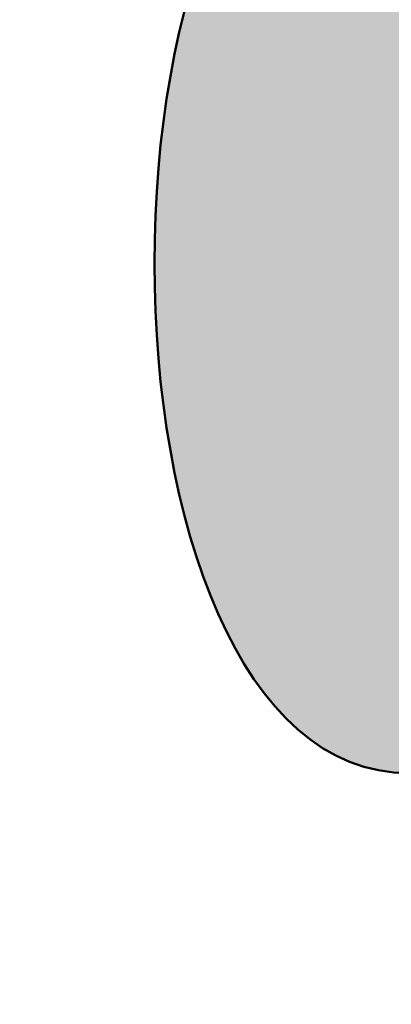
# Model space of a CAD drawing. Units: millimetres. Extents: x 0 to 2267, y 0 to 1823.
# Tile 30 of 256: x 1591.518 to 1593.341, y 1226.115 to 1230.942. Entities that reach past the tile are written whole.
import ezdxf

# ---------------------------------------------------------------- set-up
doc = ezdxf.new("R2010")
doc.units = ezdxf.units.MM
doc.header["$MEASUREMENT"] = 0
doc.layers.add('M-HATC', color=252, linetype='Continuous', lineweight=18)
doc.layers.add('M-OUTL', color=7, linetype='Continuous', lineweight=50)

msp = doc.modelspace()

# ---------------------------------------------------------------- hatches: boundary and pattern name
at = {"layer": 'M-HATC'}
h = msp.add_hatch(color=256, dxfattribs=at)
h.dxf.hatch_style = 1
h.paths.add_polyline_path([(2055.771, 1603.062), (1381.0868, 1603.062), (1381.0868, 1598.062), (2055.771, 1598.062)])
h.paths.add_polyline_path([(2055.771, 1598.062), (1381.0868, 1598.062), (1381.0868, 1593.062), (2055.771, 1593.062)])
h.paths.add_polyline_path([(2051.3074, 1536.7609), (1385.5504, 1536.7609), (1385.5504, 1526.7609), (1387.5504, 1526.7609), (1388.5366, 1525.0528), (1385.3319, 1521.2335), (1385.3319, 1521.2226), (2050.2542, 1522.7491), (2048.3212, 1525.0528), (2049.3074, 1526.7609), (2051.3074, 1526.7609)])
edge = h.paths.add_edge_path()
edge.add_arc((1847.5345, 1379.1492), 135, 222.603061, 222.890851, ccw=False)
edge.add_line((1748.1663, 1287.7656), (1683.0921, 1287.7656))
edge.add_arc((1583.7239, 1379.1492), 135, 317.109149, 317.396939, ccw=False)
edge.add_arc((1678.9686, 1290.6707), 5, 222.8909, 317.1091, ccw=False)
edge.add_arc((1774.2133, 1379.1492), 135, 222.603061, 222.890851, ccw=False)
edge.add_line((1674.8451, 1287.7656), (1609.7709, 1287.7656))
edge.add_arc((1510.4027, 1379.1492), 135, 317.109149, 317.396939, ccw=False)
edge.add_arc((1605.6474, 1290.6707), 5, 222.8909, 317.1091, ccw=False)
edge.add_arc((1700.8921, 1379.1492), 135, 222.603061, 222.890851, ccw=False)
edge.add_line((1601.5239, 1287.7656), (1536.4497, 1287.7656))
edge.add_arc((1437.0815, 1379.1492), 135, 317.109149, 317.396939, ccw=False)
edge.add_arc((1532.3262, 1290.6707), 5, 222.8909, 317.1091, ccw=False)
edge.add_arc((1627.5709, 1379.1492), 135, 222.603061, 222.890851, ccw=False)
edge.add_line((1528.2027, 1287.7656), (1505.9289, 1287.7656))
edge.add_spline(control_points=[(1505.9289, 1287.7656), (1504.2622, 1287.7656), (1504.2622, 1282.7656), (1505.9289, 1282.7656)], knot_values=[0, 0, 0, 0, 5, 5, 5, 5], degree=3, periodic=0)
edge.add_line((1505.9289, 1282.7656), (1930.9289, 1282.7656))
edge.add_spline(control_points=[(1930.9289, 1282.7656), (1932.5956, 1282.7656), (1932.5956, 1287.7656), (1930.9289, 1287.7656)], knot_values=[0, 0, 0, 0, 5, 5, 5, 5], degree=3, periodic=0)
edge.add_line((1930.9289, 1287.7656), (1903.0557, 1287.7656))
edge.add_arc((1803.6875, 1379.1492), 135, 317.109149, 317.396939, ccw=False)
edge.add_arc((1898.9322, 1290.6707), 5, 222.8909, 317.1091, ccw=False)
edge.add_arc((1994.1769, 1379.1492), 135, 222.603061, 222.890851, ccw=False)
edge.add_line((1894.8087, 1287.7656), (1829.7345, 1287.7656))
edge.add_arc((1730.3663, 1379.1492), 135, 317.109149, 317.396939, ccw=False)
edge.add_arc((1825.611, 1290.6707), 5, 222.8909, 317.1091, ccw=False)
edge.add_arc((1920.8557, 1379.1492), 135, 222.603061, 222.890851, ccw=False)
edge.add_line((1821.4875, 1287.7656), (1756.4133, 1287.7656))
edge.add_arc((1657.0451, 1379.1492), 135, 317.109149, 317.396939, ccw=False)
edge.add_arc((1752.2898, 1290.6707), 5, 222.8909, 317.1091, ccw=False)
edge = h.paths.add_edge_path()
edge.add_spline(control_points=[(1843.4289, 1227.2475), (1845.0956, 1227.2475), (1845.0956, 1232.2475), (1843.4289, 1232.2475)], knot_values=[0, 0, 0, 0, 5, 5, 5, 5], degree=3, periodic=0)
edge.add_line((1843.4289, 1232.2475), (1593.4289, 1232.2475))
edge.add_spline(control_points=[(1593.4289, 1232.2475), (1591.7622, 1232.2475), (1591.7622, 1227.2475), (1593.4289, 1227.2475)], knot_values=[0, 0, 0, 0, 5, 5, 5, 5], degree=3, periodic=0)
edge.add_line((1593.4289, 1227.2475), (1843.4289, 1227.2475))
h.paths.add_polyline_path([(1905.9289, 1127.4171), (1530.9289, 1127.4171, 0.414214), (1520.9289, 1117.4171), (1530.9289, 1117.4171), (1915.9289, 1117.4171, 0.414214)])
edge = h.paths.add_edge_path()
edge.add_arc((1397.0858, 1498.4078), 12.7299, 90.78215, 190.87871, ccw=False)
edge.add_line((1396.912, 1511.1365), (1428.0097, 1511.3488))
edge.add_line((1428.0097, 1511.3488), (1433.0097, 1511.3488))
edge.add_line((1433.0097, 1511.3488), (1434.439, 1511.3488))
edge.add_arc((1419.474, 1498.0804), 20, 41.561, 74.08211)
edge.add_line((1424.9592, 1517.3135), (1399.9351, 1517.2561))
edge.add_spline(control_points=[(1399.9307, 1517.2561), (1399.884, 1517.2131), (1399.8328, 1517.1689), (1399.7774, 1517.1236)], knot_values=[11.567499, 11.567499, 11.567499, 11.567499, 11.814249, 11.814249, 11.814249, 11.814249], degree=3, periodic=0)
edge.add_spline(control_points=[(1399.6328, 1517.0099), (1399.5831, 1516.9721), (1399.5307, 1516.9338), (1399.4759, 1516.8947)], knot_values=[11.167718, 11.167718, 11.167718, 11.167718, 11.365188, 11.365188, 11.365188, 11.365188], degree=3, periodic=0)
edge.add_spline(control_points=[(1399.3398, 1516.8001), (1399.1514, 1516.6719), (1398.9384, 1516.5377), (1398.704, 1516.3994)], knot_values=[10.376405, 10.376405, 10.376405, 10.376405, 11.00994, 11.00994, 11.00994, 11.00994], degree=3, periodic=0)
edge.add_spline(control_points=[(1398.6572, 1516.3719), (1398.5789, 1516.326), (1398.4983, 1516.2797), (1398.4155, 1516.2331)], knot_values=[10.125175, 10.125175, 10.125175, 10.125175, 10.334406, 10.334406, 10.334406, 10.334406], degree=3, periodic=0)
edge.add_spline(control_points=[(1398.2642, 1516.1487), (1398.196, 1516.1111), (1398.1263, 1516.0732), (1398.0555, 1516.0351)], knot_values=[9.832246, 9.832246, 9.832246, 9.832246, 9.999658, 9.999658, 9.999658, 9.999658], degree=3, periodic=0)
edge.add_spline(control_points=[(1397.9987, 1516.0048), (1397.7312, 1515.8621), (1397.446, 1515.7171), (1397.1466, 1515.5714)], knot_values=[9.161808, 9.161808, 9.161808, 9.161808, 9.787769, 9.787769, 9.787769, 9.787769], degree=3, periodic=0)
edge.add_spline(control_points=[(1397.1466, 1515.5714), (1396.8418, 1515.423), (1396.5222, 1515.274), (1396.1914, 1515.1262)], knot_values=[8.524455, 8.524455, 8.524455, 8.524455, 9.161808, 9.161808, 9.161808, 9.161808], degree=3, periodic=0)
edge.add_spline(control_points=[(1396.0777, 1515.0756), (1395.9854, 1515.0348), (1395.8922, 1514.994), (1395.7983, 1514.9534)], knot_values=[8.275193, 8.275193, 8.275193, 8.275193, 8.451726, 8.451726, 8.451726, 8.451726], degree=3, periodic=0)
edge.add_spline(control_points=[(1395.6018, 1514.8691), (1395.4997, 1514.8257), (1395.3968, 1514.7824), (1395.2932, 1514.7394)], knot_values=[7.962917, 7.962917, 7.962917, 7.962917, 8.152764, 8.152764, 8.152764, 8.152764], degree=3, periodic=0)
edge.add_spline(control_points=[(1395.2116, 1514.7057), (1394.8278, 1514.5475), (1394.4345, 1514.3929), (1394.0364, 1514.2442)], knot_values=[7.21254, 7.21254, 7.21254, 7.21254, 7.913148, 7.913148, 7.913148, 7.913148], degree=3, periodic=0)
edge.add_spline(control_points=[(1394.0364, 1514.2442), (1393.7076, 1514.1214), (1393.3754, 1514.0027), (1393.0427, 1513.8895)], knot_values=[6.633733, 6.633733, 6.633733, 6.633733, 7.21254, 7.21254, 7.21254, 7.21254], degree=3, periodic=0)
edge.add_spline(control_points=[(1392.8214, 1513.815), (1392.7198, 1513.7812), (1392.6181, 1513.7479), (1392.5166, 1513.7152)], knot_values=[6.328796, 6.328796, 6.328796, 6.328796, 6.505493, 6.505493, 6.505493, 6.505493], degree=3, periodic=0)
edge.add_spline(control_points=[(1392.5166, 1513.7152), (1392.3187, 1513.6515), (1392.1212, 1513.59), (1391.9244, 1513.531)], knot_values=[5.984605, 5.984605, 5.984605, 5.984605, 6.328796, 6.328796, 6.328796, 6.328796], degree=3, periodic=0)
edge.add_spline(control_points=[(1391.7915, 1513.4915), (1391.3122, 1513.3501), (1390.8384, 1513.2239), (1390.3784, 1513.1171)], knot_values=[5.066697, 5.066697, 5.066697, 5.066697, 5.907055, 5.907055, 5.907055, 5.907055], degree=3, periodic=0)
edge.add_spline(control_points=[(1390.3784, 1513.1171), (1390.1797, 1513.071), (1389.9836, 1513.0284), (1389.7907, 1512.9899)], knot_values=[4.70367, 4.70367, 4.70367, 4.70367, 5.066695, 5.066695, 5.066695, 5.066695], degree=3, periodic=0)
edge.add_spline(control_points=[(1389.422, 1512.9204), (1389.2459, 1512.8892), (1389.0729, 1512.8617), (1388.9036, 1512.8381)], knot_values=[4.130571, 4.130571, 4.130571, 4.130571, 4.469816, 4.469816, 4.469816, 4.469816], degree=3, periodic=0)
edge.add_spline(control_points=[(1388.9036, 1512.8381), (1388.591, 1512.7946), (1388.2911, 1512.7644), (1388.0071, 1512.7494)], knot_values=[3.504031, 3.504031, 3.504031, 3.504031, 4.130571, 4.130571, 4.130571, 4.130571], degree=3, periodic=0)
edge.add_spline(control_points=[(1387.9356, 1512.7459), (1387.8538, 1512.7423), (1387.7733, 1512.74), (1387.6944, 1512.739)], knot_values=[3.268866, 3.268866, 3.268866, 3.268866, 3.451164, 3.451164, 3.451164, 3.451164], degree=3, periodic=0)
edge.add_spline(control_points=[(1387.3351, 1512.7443), (1387.2076, 1512.7499), (1387.0847, 1512.7597), (1386.967, 1512.7739)], knot_values=[2.670686, 2.670686, 2.670686, 2.670686, 2.984, 2.984, 2.984, 2.984], degree=3, periodic=0)
edge.add_spline(control_points=[(1386.8327, 1512.7922), (1386.8209, 1512.7941), (1386.8092, 1512.7959), (1386.7975, 1512.7979)], knot_values=[2.516981, 2.516981, 2.516981, 2.516981, 2.549528, 2.549528, 2.549528, 2.549528], degree=3, periodic=0)
edge.add_spline(control_points=[(1386.4526, 1512.8735), (1386.4257, 1512.881), (1386.3993, 1512.889), (1386.3733, 1512.8972)], knot_values=[2.095869, 2.095869, 2.095869, 2.095869, 2.17941, 2.17941, 2.17941, 2.17941], degree=3, periodic=0)
edge.add_spline(control_points=[(1386.0691, 1513.0189), (1386.0634, 1513.0217), (1386.0577, 1513.0246), (1386.052, 1513.0275)], knot_values=[1.72453, 1.72453, 1.72453, 1.72453, 1.745933, 1.745933, 1.745933, 1.745933], degree=3, periodic=0)
edge.add_arc((1399.474, 1498.0804), 20, 131.82432, 180)
edge.add_arc((1630.3336, 1505.5484), 250.9708, 181.705176, 236.427975)
edge.add_arc((1605.3399, 1483.3044), 218.7822, 238.660829, 243.34961)
edge.add_arc((1647.0911, 1510.3592), 262.8986, 183.129836, 237.853442, ccw=False)
h.paths.add_polyline_path([(1406.5369, 1391.9644, 0.149382), (1491.5506, 1296.4418, -0.129517)], flags=17)
edge = h.paths.add_edge_path()
edge.add_arc((2037.3838, 1498.0804), 20, 0, 48.26587)
edge.add_spline(control_points=[(2050.6973, 1513.0052), (2050.6512, 1512.9847), (2050.6034, 1512.9655), (2050.5539, 1512.9477)], knot_values=[1.835652, 1.835652, 1.835652, 1.835652, 2.000781, 2.000781, 2.000781, 2.000781], degree=3, periodic=0)
edge.add_spline(control_points=[(2050.4616, 1512.9166), (2050.479, 1512.9221), (2050.4963, 1512.9277), (2050.5133, 1512.9335)], knot_values=[2.045477, 2.045477, 2.045477, 2.045477, 2.101389, 2.101389, 2.101389, 2.101389], degree=3, periodic=0)
edge.add_spline(control_points=[(2050.129, 1512.8342), (2050.1984, 1512.8473), (2050.2657, 1512.8623), (2050.3308, 1512.8792)], knot_values=[2.237629, 2.237629, 2.237629, 2.237629, 2.435841, 2.435841, 2.435841, 2.435841], degree=3, periodic=0)
edge.add_spline(control_points=[(2050.0946, 1512.8278), (2050.1061, 1512.8299), (2050.1176, 1512.832), (2050.129, 1512.8342)], knot_values=[2.435841, 2.435841, 2.435841, 2.435841, 2.468321, 2.468321, 2.468321, 2.468321], degree=3, periodic=0)
edge.add_spline(control_points=[(2049.7843, 1512.7851), (2049.8552, 1512.7922), (2049.9243, 1512.8008), (2049.9917, 1512.8109)], knot_values=[2.563852, 2.563852, 2.563852, 2.563852, 2.748541, 2.748541, 2.748541, 2.748541], degree=3, periodic=0)
edge.add_spline(control_points=[(2049.4052, 1512.7617), (2049.5364, 1512.7653), (2049.6629, 1512.773), (2049.7843, 1512.7851)], knot_values=[2.748541, 2.748541, 2.748541, 2.748541, 3.064882, 3.064882, 3.064882, 3.064882], degree=3, periodic=0)
edge.add_spline(control_points=[(2049.1698, 1512.7597), (2049.2336, 1512.7591), (2049.2965, 1512.7594), (2049.3584, 1512.7606)], knot_values=[3.102309, 3.102309, 3.102309, 3.102309, 3.2503, 3.2503, 3.2503, 3.2503], degree=3, periodic=0)
edge.add_spline(control_points=[(2048.8573, 1512.7691), (2048.9638, 1512.7638), (2049.068, 1512.7606), (2049.1698, 1512.7597)], knot_values=[3.2503, 3.2503, 3.2503, 3.2503, 3.486069, 3.486069, 3.486069, 3.486069], degree=3, periodic=0)
edge.add_spline(control_points=[(2048.6924, 1512.7789), (2048.3729, 1512.8009), (2048.0345, 1512.8411), (2047.6817, 1512.897)], knot_values=[3.606429, 3.606429, 3.606429, 3.606429, 4.2989, 4.2989, 4.2989, 4.2989], degree=3, periodic=0)
edge.add_spline(control_points=[(2047.6817, 1512.897), (2047.5458, 1512.9185), (2047.4077, 1512.9424), (2047.2678, 1512.9685)], knot_values=[4.2989, 4.2989, 4.2989, 4.2989, 4.565769, 4.565769, 4.565769, 4.565769], degree=3, periodic=0)
edge.add_spline(control_points=[(2047.2678, 1512.9685), (2047.1449, 1512.9914), (2047.0207, 1513.016), (2046.8951, 1513.0422)], knot_values=[4.565769, 4.565769, 4.565769, 4.565769, 4.799971, 4.799971, 4.799971, 4.799971], degree=3, periodic=0)
edge.add_spline(control_points=[(2046.8951, 1513.0422), (2046.5286, 1513.1188), (2046.1513, 1513.209), (2045.7676, 1513.3107)], knot_values=[4.799971, 4.799971, 4.799971, 4.799971, 5.483718, 5.483718, 5.483718, 5.483718], degree=3, periodic=0)
edge.add_spline(control_points=[(2045.7676, 1513.3107), (2045.3724, 1513.4154), (2044.9704, 1513.5322), (2044.5662, 1513.6588)], knot_values=[5.483718, 5.483718, 5.483718, 5.483718, 6.187866, 6.187866, 6.187866, 6.187866], degree=3, periodic=0)
edge.add_spline(control_points=[(2044.5662, 1513.6588), (2044.4149, 1513.7061), (2044.2633, 1513.7549), (2044.1116, 1513.8048)], knot_values=[6.187866, 6.187866, 6.187866, 6.187866, 6.451551, 6.451551, 6.451551, 6.451551], degree=3, periodic=0)
edge.add_spline(control_points=[(2044.1116, 1513.8048), (2043.9967, 1513.8427), (2043.8817, 1513.8813), (2043.7668, 1513.9205)], knot_values=[6.451551, 6.451551, 6.451551, 6.451551, 6.651434, 6.651434, 6.651434, 6.651434], degree=3, periodic=0)
edge.add_spline(control_points=[(2043.7668, 1513.9205), (2043.3716, 1514.0554), (2042.9774, 1514.1979), (2042.5886, 1514.3458)], knot_values=[6.651434, 6.651434, 6.651434, 6.651434, 7.338879, 7.338879, 7.338879, 7.338879], degree=3, periodic=0)
edge.add_spline(control_points=[(2042.5886, 1514.3458), (2042.1643, 1514.5071), (2041.7465, 1514.6749), (2041.3409, 1514.846)], knot_values=[7.338879, 7.338879, 7.338879, 7.338879, 8.089209, 8.089209, 8.089209, 8.089209], degree=3, periodic=0)
edge.add_spline(control_points=[(2041.3409, 1514.846), (2041.1028, 1514.9465), (2040.869, 1515.0481), (2040.6405, 1515.1502)], knot_values=[8.089209, 8.089209, 8.089209, 8.089209, 8.529587, 8.529587, 8.529587, 8.529587], degree=3, periodic=0)
edge.add_spline(control_points=[(2040.51, 1515.2089), (2040.0824, 1515.4022), (2039.6747, 1515.5971), (2039.295, 1515.7894)], knot_values=[8.613818, 8.613818, 8.613818, 8.613818, 9.44571, 9.44571, 9.44571, 9.44571], degree=3, periodic=0)
edge.add_spline(control_points=[(2039.295, 1515.7894), (2039.0618, 1515.9075), (2038.8391, 1516.0246), (2038.6288, 1516.1398)], knot_values=[9.44571, 9.44571, 9.44571, 9.44571, 9.956404, 9.956404, 9.956404, 9.956404], degree=3, periodic=0)
edge.add_spline(control_points=[(2038.6288, 1516.1398), (2038.5187, 1516.2001), (2038.4121, 1516.2598), (2038.309, 1516.3189)], knot_values=[9.956404, 9.956404, 9.956404, 9.956404, 10.223542, 10.223542, 10.223542, 10.223542], degree=3, periodic=0)
edge.add_spline(control_points=[(2038.309, 1516.3189), (2038.2138, 1516.3735), (2038.1216, 1516.4276), (2038.0328, 1516.481)], knot_values=[10.223542, 10.223542, 10.223542, 10.223542, 10.47051, 10.47051, 10.47051, 10.47051], degree=3, periodic=0)
edge.add_spline(control_points=[(2038.0328, 1516.481), (2037.7855, 1516.6296), (2037.5639, 1516.773), (2037.3722, 1516.909)], knot_values=[10.47051, 10.47051, 10.47051, 10.47051, 11.15767, 11.15767, 11.15767, 11.15767], degree=3, periodic=0)
edge.add_spline(control_points=[(2037.3722, 1516.909), (2037.2789, 1516.9752), (2037.1927, 1517.0396), (2037.1142, 1517.102)], knot_values=[11.15767, 11.15767, 11.15767, 11.15767, 11.49227, 11.49227, 11.49227, 11.49227], degree=3, periodic=0)
edge.add_spline(control_points=[(2036.8564, 1517.3259), (2036.9148, 1517.2692), (2036.9814, 1517.2103), (2037.0557, 1517.1492)], knot_values=[11.577341, 11.577341, 11.577341, 11.577341, 11.91035, 11.91035, 11.91035, 11.91035], degree=3, periodic=0)
edge.add_spline(control_points=[(2036.8074, 1517.3748), (2036.823, 1517.3587), (2036.8393, 1517.3424), (2036.8564, 1517.3259)], knot_values=[11.91035, 11.91035, 11.91035, 11.91035, 12.007402, 12.007402, 12.007402, 12.007402], degree=3, periodic=0)
edge.add_spline(control_points=[(2036.7017, 1517.494), (2036.7104, 1517.483), (2036.7196, 1517.4719), (2036.7291, 1517.4606)], knot_values=[12.184155, 12.184155, 12.184155, 12.184155, 12.255409, 12.255409, 12.255409, 12.255409], degree=3, periodic=0)
edge.add_spline(control_points=[(2036.6159, 1517.6205), (2036.62, 1517.613), (2036.6243, 1517.6055), (2036.6289, 1517.5979)], knot_values=[12.487913, 12.487913, 12.487913, 12.487913, 12.541035, 12.541035, 12.541035, 12.541035], degree=3, periodic=0)
edge.add_spline(control_points=[(2036.5635, 1517.786), (2036.5637, 1517.7794), (2036.5642, 1517.7726), (2036.565, 1517.7658)], knot_values=[12.911761, 12.911761, 12.911761, 12.911761, 12.968286, 12.968286, 12.968286, 12.968286], degree=3, periodic=0)
edge.add_spline(control_points=[(2036.6166, 1517.9304), (2036.6125, 1517.9259), (2036.6086, 1517.9212), (2036.6049, 1517.9165)], knot_values=[13.382527, 13.382527, 13.382527, 13.382527, 13.433791, 13.433791, 13.433791, 13.433791], degree=3, periodic=0)
edge.add_spline(control_points=[(2036.749, 1518.017), (2036.7361, 1518.0116), (2036.7239, 1518.006), (2036.7124, 1518.0002)], knot_values=[13.726299, 13.726299, 13.726299, 13.726299, 13.809928, 13.809928, 13.809928, 13.809928], degree=3, periodic=0)
edge.add_spline(control_points=[(2036.8604, 1518.0528), (2036.8386, 1518.0474), (2036.8181, 1518.0416), (2036.7988, 1518.0353)], knot_values=[13.910887, 13.910887, 13.910887, 13.910887, 14.02153, 14.02153, 14.02153, 14.02153], degree=3, periodic=0)
edge.add_line((2036.9639, 1518.0804), (2032.3838, 1518.0804))
edge.add_line((2032.3838, 1518.0804), (2027.3838, 1518.0804))
edge.add_line((2027.3838, 1518.0804), (2022.3838, 1518.0804))
edge.add_line((2022.3838, 1518.0804), (2017.3838, 1518.0804))
edge.add_arc((2017.3838, 1498.0804), 20, 90, 138.439)
edge.add_line((2002.4188, 1511.3488), (2003.8481, 1511.3488))
edge.add_line((2003.8481, 1511.3488), (2008.8481, 1511.3488))
edge.add_line((2008.8481, 1511.3488), (2039.772, 1511.1377))
edge.add_arc((2039.772, 1498.4078), 12.7299, -10.87871, 90, ccw=False)
edge.add_arc((1789.7668, 1510.3592), 262.8986, 302.146558, 356.870164, ccw=False)
edge.add_arc((1831.5179, 1483.3044), 218.7822, 296.65039, 301.339171)
edge.add_arc((1806.5242, 1505.5484), 250.9708, 303.572025, 358.294824)
h.paths.add_polyline_path([(2030.321, 1391.9644, -0.129517), (1945.3072, 1296.4418, 0.149382)], flags=17)
edge = h.paths.add_edge_path()
edge.add_spline(control_points=[(2037.2464, 1518.0821), (2037.2898, 1518.081), (2037.3355, 1518.0804), (2037.3838, 1518.0804)], knot_values=[0.000012, 0.000012, 0.000012, 0.000012, 0.144754, 0.144754, 0.144754, 0.144754], degree=3, periodic=0)
edge.add_line((2037.3357, 1518.0804), (2037.0096, 1518.0804))
edge.add_spline(control_points=[(2037.0096, 1518.0804), (2036.9822, 1518.0768), (2036.956, 1518.0727), (2036.9312, 1518.0681)], knot_values=[14.13465, 14.13465, 14.13465, 14.13465, 14.247197, 14.247197, 14.247197, 14.247197], degree=3, periodic=0)
edge.add_spline(control_points=[(2036.9312, 1518.0681), (2036.9276, 1518.0674), (2036.9241, 1518.0667), (2036.9205, 1518.0661)], knot_values=[14.118315, 14.118315, 14.118315, 14.118315, 14.13465, 14.13465, 14.13465, 14.13465], degree=3, periodic=0)
edge.add_spline(control_points=[(2036.9205, 1518.0661), (2036.9118, 1518.0644), (2036.9032, 1518.0626), (2036.8948, 1518.0608)], knot_values=[14.078086, 14.078086, 14.078086, 14.078086, 14.118315, 14.118315, 14.118315, 14.118315], degree=3, periodic=0)
edge.add_spline(control_points=[(2036.8948, 1518.0608), (2036.883, 1518.0583), (2036.8716, 1518.0556), (2036.8604, 1518.0528)], knot_values=[14.02153, 14.02153, 14.02153, 14.02153, 14.078086, 14.078086, 14.078086, 14.078086], degree=3, periodic=0)
edge.add_spline(control_points=[(2036.8604, 1518.0528), (2036.8386, 1518.0474), (2036.8181, 1518.0416), (2036.7988, 1518.0353)], knot_values=[13.910887, 13.910887, 13.910887, 13.910887, 14.02153, 14.02153, 14.02153, 14.02153], degree=3, periodic=0)
edge.add_spline(control_points=[(2036.7988, 1518.0353), (2036.7981, 1518.035), (2036.7974, 1518.0348), (2036.7967, 1518.0346)], knot_values=[13.906906, 13.906906, 13.906906, 13.906906, 13.910887, 13.910887, 13.910887, 13.910887], degree=3, periodic=0)
edge.add_spline(control_points=[(2036.7967, 1518.0346), (2036.7882, 1518.0318), (2036.7799, 1518.0289), (2036.7719, 1518.0259)], knot_values=[13.857826, 13.857826, 13.857826, 13.857826, 13.906906, 13.906906, 13.906906, 13.906906], degree=3, periodic=0)
edge.add_spline(control_points=[(2036.7719, 1518.0259), (2036.764, 1518.023), (2036.7564, 1518.02), (2036.749, 1518.017)], knot_values=[13.809928, 13.809928, 13.809928, 13.809928, 13.857826, 13.857826, 13.857826, 13.857826], degree=3, periodic=0)
edge.add_spline(control_points=[(2036.749, 1518.017), (2036.7361, 1518.0116), (2036.7239, 1518.006), (2036.7124, 1518.0002)], knot_values=[13.726299, 13.726299, 13.726299, 13.726299, 13.809928, 13.809928, 13.809928, 13.809928], degree=3, periodic=0)
edge.add_spline(control_points=[(2036.7124, 1518.0002), (2036.7121, 1518), (2036.7118, 1517.9999), (2036.7115, 1517.9997)], knot_values=[13.723993, 13.723993, 13.723993, 13.723993, 13.726299, 13.726299, 13.726299, 13.726299], degree=3, periodic=0)
edge.add_spline(control_points=[(2036.7115, 1517.9997), (2036.7063, 1517.9971), (2036.7013, 1517.9944), (2036.6965, 1517.9917)], knot_values=[13.686536, 13.686536, 13.686536, 13.686536, 13.723993, 13.723993, 13.723993, 13.723993], degree=3, periodic=0)
edge.add_spline(control_points=[(2036.6965, 1517.9917), (2036.6919, 1517.9891), (2036.6874, 1517.9865), (2036.6831, 1517.9839)], knot_values=[13.651251, 13.651251, 13.651251, 13.651251, 13.686536, 13.686536, 13.686536, 13.686536], degree=3, periodic=0)
edge.add_spline(control_points=[(2036.6831, 1517.9839), (2036.6764, 1517.9798), (2036.67, 1517.9757), (2036.6639, 1517.9714)], knot_values=[13.596804, 13.596804, 13.596804, 13.596804, 13.651251, 13.651251, 13.651251, 13.651251], degree=3, periodic=0)
edge.add_spline(control_points=[(2036.6639, 1517.9714), (2036.6636, 1517.9712), (2036.6633, 1517.9709), (2036.6629, 1517.9707)], knot_values=[13.593956, 13.593956, 13.593956, 13.593956, 13.596804, 13.596804, 13.596804, 13.596804], degree=3, periodic=0)
edge.add_spline(control_points=[(2036.6629, 1517.9707), (2036.6603, 1517.9689), (2036.6577, 1517.967), (2036.6552, 1517.9651)], knot_values=[13.570322, 13.570322, 13.570322, 13.570322, 13.593956, 13.593956, 13.593956, 13.593956], degree=3, periodic=0)
edge.add_spline(control_points=[(2036.6552, 1517.9651), (2036.6525, 1517.9631), (2036.6499, 1517.9611), (2036.6474, 1517.9591)], knot_values=[13.545477, 13.545477, 13.545477, 13.545477, 13.570322, 13.570322, 13.570322, 13.570322], degree=3, periodic=0)
edge.add_spline(control_points=[(2036.6474, 1517.9591), (2036.6472, 1517.9589), (2036.6471, 1517.9588), (2036.6469, 1517.9587)], knot_values=[13.543931, 13.543931, 13.543931, 13.543931, 13.545477, 13.545477, 13.545477, 13.545477], degree=3, periodic=0)
edge.add_spline(control_points=[(2036.6469, 1517.9587), (2036.6412, 1517.9541), (2036.6358, 1517.9494), (2036.6307, 1517.9447)], knot_values=[13.488237, 13.488237, 13.488237, 13.488237, 13.543931, 13.543931, 13.543931, 13.543931], degree=3, periodic=0)
edge.add_spline(control_points=[(2036.6307, 1517.9447), (2036.6282, 1517.9423), (2036.6257, 1517.9399), (2036.6233, 1517.9374)], knot_values=[13.460307, 13.460307, 13.460307, 13.460307, 13.488237, 13.488237, 13.488237, 13.488237], degree=3, periodic=0)
edge.add_spline(control_points=[(2036.6233, 1517.9374), (2036.6215, 1517.9356), (2036.6198, 1517.9338), (2036.6181, 1517.932)], knot_values=[13.439712, 13.439712, 13.439712, 13.439712, 13.460307, 13.460307, 13.460307, 13.460307], degree=3, periodic=0)
edge.add_spline(control_points=[(2036.6181, 1517.932), (2036.6176, 1517.9315), (2036.6171, 1517.9309), (2036.6166, 1517.9304)], knot_values=[13.433791, 13.433791, 13.433791, 13.433791, 13.439712, 13.439712, 13.439712, 13.439712], degree=3, periodic=0)
edge.add_spline(control_points=[(2036.6166, 1517.9304), (2036.6125, 1517.9259), (2036.6086, 1517.9212), (2036.6049, 1517.9165)], knot_values=[13.382527, 13.382527, 13.382527, 13.382527, 13.433791, 13.433791, 13.433791, 13.433791], degree=3, periodic=0)
edge.add_spline(control_points=[(2036.6049, 1517.9165), (2036.6026, 1517.9135), (2036.6004, 1517.9104), (2036.5982, 1517.9074)], knot_values=[13.350017, 13.350017, 13.350017, 13.350017, 13.382527, 13.382527, 13.382527, 13.382527], degree=3, periodic=0)
edge.add_spline(control_points=[(2036.5982, 1517.9074), (2036.5972, 1517.9059), (2036.5962, 1517.9043), (2036.5952, 1517.9028)], knot_values=[13.333922, 13.333922, 13.333922, 13.333922, 13.350017, 13.350017, 13.350017, 13.350017], degree=3, periodic=0)
edge.add_spline(control_points=[(2036.5952, 1517.9028), (2036.5945, 1517.9018), (2036.5939, 1517.9009), (2036.5933, 1517.8999)], knot_values=[13.323828, 13.323828, 13.323828, 13.323828, 13.333922, 13.333922, 13.333922, 13.333922], degree=3, periodic=0)
edge.add_spline(control_points=[(2036.5933, 1517.8999), (2036.5905, 1517.8955), (2036.5879, 1517.8909), (2036.5855, 1517.8864)], knot_values=[13.277545, 13.277545, 13.277545, 13.277545, 13.323828, 13.323828, 13.323828, 13.323828], degree=3, periodic=0)
edge.add_spline(control_points=[(2036.5855, 1517.8864), (2036.5836, 1517.8827), (2036.5817, 1517.8789), (2036.5801, 1517.8751)], knot_values=[13.240119, 13.240119, 13.240119, 13.240119, 13.277545, 13.277545, 13.277545, 13.277545], degree=3, periodic=0)
edge.add_spline(control_points=[(2036.5801, 1517.8751), (2036.5795, 1517.8739), (2036.579, 1517.8727), (2036.5785, 1517.8715)], knot_values=[13.228211, 13.228211, 13.228211, 13.228211, 13.240119, 13.240119, 13.240119, 13.240119], degree=3, periodic=0)
edge.add_spline(control_points=[(2036.5785, 1517.8715), (2036.578, 1517.8702), (2036.5774, 1517.869), (2036.5769, 1517.8677)], knot_values=[13.215717, 13.215717, 13.215717, 13.215717, 13.228211, 13.228211, 13.228211, 13.228211], degree=3, periodic=0)
edge.add_spline(control_points=[(2036.5769, 1517.8677), (2036.5755, 1517.864), (2036.5741, 1517.8603), (2036.5729, 1517.8565)], knot_values=[13.179847, 13.179847, 13.179847, 13.179847, 13.215717, 13.215717, 13.215717, 13.215717], degree=3, periodic=0)
edge.add_spline(control_points=[(2036.5729, 1517.8565), (2036.5713, 1517.8515), (2036.5699, 1517.8464), (2036.5687, 1517.8413)], knot_values=[13.132017, 13.132017, 13.132017, 13.132017, 13.179847, 13.179847, 13.179847, 13.179847], degree=3, periodic=0)
edge.add_spline(control_points=[(2036.5687, 1517.8413), (2036.5684, 1517.8402), (2036.5682, 1517.8392), (2036.568, 1517.8382)], knot_values=[13.122482, 13.122482, 13.122482, 13.122482, 13.132017, 13.132017, 13.132017, 13.132017], degree=3, periodic=0)
edge.add_spline(control_points=[(2036.568, 1517.8382), (2036.5676, 1517.8363), (2036.5672, 1517.8345), (2036.5669, 1517.8327)], knot_values=[13.105592, 13.105592, 13.105592, 13.105592, 13.122482, 13.122482, 13.122482, 13.122482], degree=3, periodic=0)
edge.add_spline(control_points=[(2036.5669, 1517.8327), (2036.5662, 1517.8292), (2036.5657, 1517.8257), (2036.5652, 1517.8222)], knot_values=[13.074063, 13.074063, 13.074063, 13.074063, 13.105592, 13.105592, 13.105592, 13.105592], degree=3, periodic=0)
edge.add_spline(control_points=[(2036.5652, 1517.8222), (2036.5652, 1517.8222), (2036.5652, 1517.8222), (2036.5652, 1517.8222)], knot_values=[13.074043, 13.074043, 13.074043, 13.074043, 13.074063, 13.074063, 13.074063, 13.074063], degree=3, periodic=0)
edge.add_spline(control_points=[(2036.5652, 1517.8222), (2036.5644, 1517.8164), (2036.5639, 1517.8106), (2036.5636, 1517.8046)], knot_values=[13.021884, 13.021884, 13.021884, 13.021884, 13.074043, 13.074043, 13.074043, 13.074043], degree=3, periodic=0)
edge.add_spline(control_points=[(2036.5636, 1517.8046), (2036.5636, 1517.804), (2036.5636, 1517.8034), (2036.5635, 1517.8028)], knot_values=[13.01674, 13.01674, 13.01674, 13.01674, 13.021884, 13.021884, 13.021884, 13.021884], degree=3, periodic=0)
edge.add_spline(control_points=[(2036.5635, 1517.8028), (2036.5634, 1517.8005), (2036.5634, 1517.7982), (2036.5634, 1517.7958)], knot_values=[12.996438, 12.996438, 12.996438, 12.996438, 13.01674, 13.01674, 13.01674, 13.01674], degree=3, periodic=0)
edge.add_spline(control_points=[(2036.5634, 1517.7958), (2036.5633, 1517.7926), (2036.5634, 1517.7893), (2036.5635, 1517.786)], knot_values=[12.968286, 12.968286, 12.968286, 12.968286, 12.996438, 12.996438, 12.996438, 12.996438], degree=3, periodic=0)
edge.add_spline(control_points=[(2036.5635, 1517.786), (2036.5637, 1517.7794), (2036.5642, 1517.7726), (2036.565, 1517.7658)], knot_values=[12.911761, 12.911761, 12.911761, 12.911761, 12.968286, 12.968286, 12.968286, 12.968286], degree=3, periodic=0)
edge.add_spline(control_points=[(2036.565, 1517.7658), (2036.565, 1517.7657), (2036.565, 1517.7656), (2036.565, 1517.7656)], knot_values=[12.911017, 12.911017, 12.911017, 12.911017, 12.911761, 12.911761, 12.911761, 12.911761], degree=3, periodic=0)
edge.add_spline(control_points=[(2036.565, 1517.7656), (2036.5654, 1517.7625), (2036.5658, 1517.7593), (2036.5663, 1517.7562)], knot_values=[12.88528, 12.88528, 12.88528, 12.88528, 12.911017, 12.911017, 12.911017, 12.911017], degree=3, periodic=0)
edge.add_spline(control_points=[(2036.5663, 1517.7562), (2036.5667, 1517.7534), (2036.5672, 1517.7506), (2036.5677, 1517.7478)], knot_values=[12.862519, 12.862519, 12.862519, 12.862519, 12.88528, 12.88528, 12.88528, 12.88528], degree=3, periodic=0)
edge.add_spline(control_points=[(2036.5677, 1517.7478), (2036.5678, 1517.7474), (2036.5679, 1517.7469), (2036.568, 1517.7465)], knot_values=[12.858885, 12.858885, 12.858885, 12.858885, 12.862519, 12.862519, 12.862519, 12.862519], degree=3, periodic=0)
edge.add_spline(control_points=[(2036.568, 1517.7465), (2036.5692, 1517.7399), (2036.5707, 1517.7332), (2036.5724, 1517.7264)], knot_values=[12.8053, 12.8053, 12.8053, 12.8053, 12.858885, 12.858885, 12.858885, 12.858885], degree=3, periodic=0)
edge.add_spline(control_points=[(2036.5724, 1517.7264), (2036.5734, 1517.7226), (2036.5745, 1517.7187), (2036.5756, 1517.7149)], knot_values=[12.775176, 12.775176, 12.775176, 12.775176, 12.8053, 12.8053, 12.8053, 12.8053], degree=3, periodic=0)
edge.add_spline(control_points=[(2036.5756, 1517.7149), (2036.5763, 1517.7125), (2036.577, 1517.7102), (2036.5778, 1517.7078)], knot_values=[12.756759, 12.756759, 12.756759, 12.756759, 12.775176, 12.775176, 12.775176, 12.775176], degree=3, periodic=0)
edge.add_spline(control_points=[(2036.5778, 1517.7078), (2036.5781, 1517.7067), (2036.5784, 1517.7057), (2036.5787, 1517.7047)], knot_values=[12.748742, 12.748742, 12.748742, 12.748742, 12.756759, 12.756759, 12.756759, 12.756759], degree=3, periodic=0)
edge.add_spline(control_points=[(2036.5787, 1517.7047), (2036.5808, 1517.6983), (2036.5831, 1517.6919), (2036.5856, 1517.6854)], knot_values=[12.69959, 12.69959, 12.69959, 12.69959, 12.748742, 12.748742, 12.748742, 12.748742], degree=3, periodic=0)
edge.add_spline(control_points=[(2036.5856, 1517.6854), (2036.5876, 1517.68), (2036.5898, 1517.6746), (2036.5921, 1517.6692)], knot_values=[12.659038, 12.659038, 12.659038, 12.659038, 12.69959, 12.69959, 12.69959, 12.69959], degree=3, periodic=0)
edge.add_spline(control_points=[(2036.5921, 1517.6692), (2036.594, 1517.6648), (2036.5959, 1517.6605), (2036.5979, 1517.6561)], knot_values=[12.626806, 12.626806, 12.626806, 12.626806, 12.659038, 12.659038, 12.659038, 12.659038], degree=3, periodic=0)
edge.add_spline(control_points=[(2036.5979, 1517.6561), (2036.5984, 1517.6551), (2036.5989, 1517.6541), (2036.5993, 1517.6531)], knot_values=[12.619394, 12.619394, 12.619394, 12.619394, 12.626806, 12.626806, 12.626806, 12.626806], degree=3, periodic=0)
edge.add_spline(control_points=[(2036.5993, 1517.6531), (2036.6043, 1517.6424), (2036.6099, 1517.6315), (2036.6159, 1517.6205)], knot_values=[12.541039, 12.541039, 12.541039, 12.541039, 12.619394, 12.619394, 12.619394, 12.619394], degree=3, periodic=0)
edge.add_spline(control_points=[(2036.6159, 1517.6205), (2036.6159, 1517.6205), (2036.6159, 1517.6205), (2036.6159, 1517.6205)], knot_values=[12.541035, 12.541035, 12.541035, 12.541035, 12.541039, 12.541039, 12.541039, 12.541039], degree=3, periodic=0)
edge.add_spline(control_points=[(2036.6159, 1517.6205), (2036.62, 1517.613), (2036.6243, 1517.6055), (2036.6289, 1517.5979)], knot_values=[12.487913, 12.487913, 12.487913, 12.487913, 12.541035, 12.541035, 12.541035, 12.541035], degree=3, periodic=0)
edge.add_spline(control_points=[(2036.6289, 1517.5979), (2036.6326, 1517.5916), (2036.6365, 1517.5853), (2036.6406, 1517.5789)], knot_values=[12.443982, 12.443982, 12.443982, 12.443982, 12.487913, 12.487913, 12.487913, 12.487913], degree=3, periodic=0)
edge.add_spline(control_points=[(2036.6406, 1517.5789), (2036.6414, 1517.5776), (2036.6423, 1517.5763), (2036.6431, 1517.5749)], knot_values=[12.434996, 12.434996, 12.434996, 12.434996, 12.443982, 12.443982, 12.443982, 12.443982], degree=3, periodic=0)
edge.add_spline(control_points=[(2036.6431, 1517.5749), (2036.6531, 1517.5596), (2036.6639, 1517.5439), (2036.6756, 1517.528)], knot_values=[12.329647, 12.329647, 12.329647, 12.329647, 12.434996, 12.434996, 12.434996, 12.434996], degree=3, periodic=0)
edge.add_spline(control_points=[(2036.6756, 1517.528), (2036.6839, 1517.5168), (2036.6925, 1517.5055), (2036.7017, 1517.494)], knot_values=[12.255409, 12.255409, 12.255409, 12.255409, 12.329647, 12.329647, 12.329647, 12.329647], degree=3, periodic=0)
edge.add_spline(control_points=[(2036.7017, 1517.494), (2036.7104, 1517.483), (2036.7196, 1517.4719), (2036.7291, 1517.4606)], knot_values=[12.184155, 12.184155, 12.184155, 12.184155, 12.255409, 12.255409, 12.255409, 12.255409], degree=3, periodic=0)
edge.add_spline(control_points=[(2036.7291, 1517.4606), (2036.7436, 1517.4435), (2036.759, 1517.4262), (2036.7753, 1517.4085)], knot_values=[12.075961, 12.075961, 12.075961, 12.075961, 12.184155, 12.184155, 12.184155, 12.184155], degree=3, periodic=0)
edge.add_spline(control_points=[(2036.7753, 1517.4085), (2036.7763, 1517.4075), (2036.7773, 1517.4064), (2036.7783, 1517.4054)], knot_values=[12.069502, 12.069502, 12.069502, 12.069502, 12.075961, 12.075961, 12.075961, 12.075961], degree=3, periodic=0)
edge.add_spline(control_points=[(2036.7783, 1517.4054), (2036.7877, 1517.3953), (2036.7974, 1517.385), (2036.8074, 1517.3748)], knot_values=[12.007402, 12.007402, 12.007402, 12.007402, 12.069502, 12.069502, 12.069502, 12.069502], degree=3, periodic=0)
edge.add_spline(control_points=[(2036.8074, 1517.3748), (2036.823, 1517.3587), (2036.8393, 1517.3424), (2036.8564, 1517.3259)], knot_values=[11.91035, 11.91035, 11.91035, 11.91035, 12.007402, 12.007402, 12.007402, 12.007402], degree=3, periodic=0)
edge.add_spline(control_points=[(2036.8564, 1517.3259), (2036.9148, 1517.2692), (2036.9814, 1517.2103), (2037.0557, 1517.1492)], knot_values=[11.577341, 11.577341, 11.577341, 11.577341, 11.91035, 11.91035, 11.91035, 11.91035], degree=3, periodic=0)
edge.add_spline(control_points=[(2037.0557, 1517.1492), (2037.0747, 1517.1336), (2037.0942, 1517.1179), (2037.1142, 1517.102)], knot_values=[11.49227, 11.49227, 11.49227, 11.49227, 11.577341, 11.577341, 11.577341, 11.577341], degree=3, periodic=0)
edge.add_spline(control_points=[(2037.1142, 1517.102), (2037.1927, 1517.0396), (2037.2789, 1516.9752), (2037.3722, 1516.909)], knot_values=[11.15767, 11.15767, 11.15767, 11.15767, 11.49227, 11.49227, 11.49227, 11.49227], degree=3, periodic=0)
edge.add_spline(control_points=[(2037.3722, 1516.909), (2037.5639, 1516.773), (2037.7855, 1516.6296), (2038.0328, 1516.481)], knot_values=[10.47051, 10.47051, 10.47051, 10.47051, 11.15767, 11.15767, 11.15767, 11.15767], degree=3, periodic=0)
edge.add_spline(control_points=[(2038.0328, 1516.481), (2038.1216, 1516.4276), (2038.2138, 1516.3735), (2038.309, 1516.3189)], knot_values=[10.223542, 10.223542, 10.223542, 10.223542, 10.47051, 10.47051, 10.47051, 10.47051], degree=3, periodic=0)
edge.add_spline(control_points=[(2038.309, 1516.3189), (2038.4121, 1516.2598), (2038.5187, 1516.2001), (2038.6288, 1516.1398)], knot_values=[9.956404, 9.956404, 9.956404, 9.956404, 10.223542, 10.223542, 10.223542, 10.223542], degree=3, periodic=0)
edge.add_spline(control_points=[(2038.6288, 1516.1398), (2038.8391, 1516.0246), (2039.0618, 1515.9075), (2039.295, 1515.7894)], knot_values=[9.44571, 9.44571, 9.44571, 9.44571, 9.956404, 9.956404, 9.956404, 9.956404], degree=3, periodic=0)
edge.add_spline(control_points=[(2039.295, 1515.7894), (2039.6747, 1515.5971), (2040.0824, 1515.4022), (2040.51, 1515.2089)], knot_values=[8.613818, 8.613818, 8.613818, 8.613818, 9.44571, 9.44571, 9.44571, 9.44571], degree=3, periodic=0)
edge.add_spline(control_points=[(2040.51, 1515.2089), (2040.5533, 1515.1893), (2040.5968, 1515.1697), (2040.6405, 1515.1502)], knot_values=[8.529587, 8.529587, 8.529587, 8.529587, 8.613818, 8.613818, 8.613818, 8.613818], degree=3, periodic=0)
edge.add_spline(control_points=[(2040.6405, 1515.1502), (2040.869, 1515.0481), (2041.1028, 1514.9465), (2041.3409, 1514.846)], knot_values=[8.089209, 8.089209, 8.089209, 8.089209, 8.529587, 8.529587, 8.529587, 8.529587], degree=3, periodic=0)
edge.add_spline(control_points=[(2041.3409, 1514.846), (2041.7465, 1514.6749), (2042.1643, 1514.5071), (2042.5886, 1514.3458)], knot_values=[7.338879, 7.338879, 7.338879, 7.338879, 8.089209, 8.089209, 8.089209, 8.089209], degree=3, periodic=0)
edge.add_spline(control_points=[(2042.5886, 1514.3458), (2042.9774, 1514.1979), (2043.3716, 1514.0554), (2043.7668, 1513.9205)], knot_values=[6.651434, 6.651434, 6.651434, 6.651434, 7.338879, 7.338879, 7.338879, 7.338879], degree=3, periodic=0)
edge.add_spline(control_points=[(2043.7668, 1513.9205), (2043.8817, 1513.8813), (2043.9967, 1513.8427), (2044.1116, 1513.8048)], knot_values=[6.451551, 6.451551, 6.451551, 6.451551, 6.651434, 6.651434, 6.651434, 6.651434], degree=3, periodic=0)
edge.add_spline(control_points=[(2044.1116, 1513.8048), (2044.2633, 1513.7549), (2044.4149, 1513.7061), (2044.5662, 1513.6588)], knot_values=[6.187866, 6.187866, 6.187866, 6.187866, 6.451551, 6.451551, 6.451551, 6.451551], degree=3, periodic=0)
edge.add_spline(control_points=[(2044.5662, 1513.6588), (2044.9704, 1513.5322), (2045.3724, 1513.4154), (2045.7676, 1513.3107)], knot_values=[5.483718, 5.483718, 5.483718, 5.483718, 6.187866, 6.187866, 6.187866, 6.187866], degree=3, periodic=0)
edge.add_spline(control_points=[(2045.7676, 1513.3107), (2046.1513, 1513.209), (2046.5286, 1513.1188), (2046.8951, 1513.0422)], knot_values=[4.799971, 4.799971, 4.799971, 4.799971, 5.483718, 5.483718, 5.483718, 5.483718], degree=3, periodic=0)
edge.add_spline(control_points=[(2046.8951, 1513.0422), (2047.0207, 1513.016), (2047.1449, 1512.9914), (2047.2678, 1512.9685)], knot_values=[4.565769, 4.565769, 4.565769, 4.565769, 4.799971, 4.799971, 4.799971, 4.799971], degree=3, periodic=0)
edge.add_spline(control_points=[(2047.2678, 1512.9685), (2047.4077, 1512.9424), (2047.5458, 1512.9185), (2047.6817, 1512.897)], knot_values=[4.2989, 4.2989, 4.2989, 4.2989, 4.565769, 4.565769, 4.565769, 4.565769], degree=3, periodic=0)
edge.add_spline(control_points=[(2047.6817, 1512.897), (2048.0345, 1512.8411), (2048.3729, 1512.8009), (2048.6924, 1512.7789)], knot_values=[3.606429, 3.606429, 3.606429, 3.606429, 4.2989, 4.2989, 4.2989, 4.2989], degree=3, periodic=0)
edge.add_spline(control_points=[(2048.6924, 1512.7789), (2048.7479, 1512.7751), (2048.8029, 1512.7718), (2048.8573, 1512.7691)], knot_values=[3.486069, 3.486069, 3.486069, 3.486069, 3.606429, 3.606429, 3.606429, 3.606429], degree=3, periodic=0)
edge.add_spline(control_points=[(2048.8573, 1512.7691), (2048.9638, 1512.7638), (2049.068, 1512.7606), (2049.1698, 1512.7597)], knot_values=[3.2503, 3.2503, 3.2503, 3.2503, 3.486069, 3.486069, 3.486069, 3.486069], degree=3, periodic=0)
edge.add_spline(control_points=[(2049.1698, 1512.7597), (2049.2336, 1512.7591), (2049.2965, 1512.7594), (2049.3584, 1512.7606)], knot_values=[3.102309, 3.102309, 3.102309, 3.102309, 3.2503, 3.2503, 3.2503, 3.2503], degree=3, periodic=0)
edge.add_spline(control_points=[(2049.3584, 1512.7606), (2049.3741, 1512.7609), (2049.3897, 1512.7613), (2049.4052, 1512.7617)], knot_values=[3.064882, 3.064882, 3.064882, 3.064882, 3.102309, 3.102309, 3.102309, 3.102309], degree=3, periodic=0)
edge.add_spline(control_points=[(2049.4052, 1512.7617), (2049.5364, 1512.7653), (2049.6629, 1512.773), (2049.7843, 1512.7851)], knot_values=[2.748541, 2.748541, 2.748541, 2.748541, 3.064882, 3.064882, 3.064882, 3.064882], degree=3, periodic=0)
edge.add_spline(control_points=[(2049.7843, 1512.7851), (2049.8552, 1512.7922), (2049.9243, 1512.8008), (2049.9917, 1512.8109)], knot_values=[2.563852, 2.563852, 2.563852, 2.563852, 2.748541, 2.748541, 2.748541, 2.748541], degree=3, periodic=0)
edge.add_spline(control_points=[(2049.9917, 1512.8109), (2050.0265, 1512.8161), (2050.0608, 1512.8218), (2050.0946, 1512.8278)], knot_values=[2.468321, 2.468321, 2.468321, 2.468321, 2.563852, 2.563852, 2.563852, 2.563852], degree=3, periodic=0)
edge.add_spline(control_points=[(2050.0946, 1512.8278), (2050.1061, 1512.8299), (2050.1176, 1512.832), (2050.129, 1512.8342)], knot_values=[2.435841, 2.435841, 2.435841, 2.435841, 2.468321, 2.468321, 2.468321, 2.468321], degree=3, periodic=0)
edge.add_spline(control_points=[(2050.129, 1512.8342), (2050.1984, 1512.8473), (2050.2657, 1512.8623), (2050.3308, 1512.8792)], knot_values=[2.237629, 2.237629, 2.237629, 2.237629, 2.435841, 2.435841, 2.435841, 2.435841], degree=3, periodic=0)
edge.add_spline(control_points=[(2050.3308, 1512.8792), (2050.3754, 1512.8908), (2050.4191, 1512.9032), (2050.4616, 1512.9166)], knot_values=[2.101389, 2.101389, 2.101389, 2.101389, 2.237629, 2.237629, 2.237629, 2.237629], degree=3, periodic=0)
edge.add_spline(control_points=[(2050.4616, 1512.9166), (2050.479, 1512.9221), (2050.4963, 1512.9277), (2050.5133, 1512.9335)], knot_values=[2.045477, 2.045477, 2.045477, 2.045477, 2.101389, 2.101389, 2.101389, 2.101389], degree=3, periodic=0)
edge.add_spline(control_points=[(2050.5133, 1512.9335), (2050.527, 1512.9382), (2050.5405, 1512.9429), (2050.5539, 1512.9477)], knot_values=[2.000781, 2.000781, 2.000781, 2.000781, 2.045477, 2.045477, 2.045477, 2.045477], degree=3, periodic=0)
edge.add_spline(control_points=[(2050.5539, 1512.9477), (2050.6034, 1512.9655), (2050.6512, 1512.9847), (2050.6973, 1513.0052)], knot_values=[1.835652, 1.835652, 1.835652, 1.835652, 2.000781, 2.000781, 2.000781, 2.000781], degree=3, periodic=0)
edge.add_arc((2037.3838, 1498.0804), 20, 48.26587, 90.12993)
edge = h.paths.add_edge_path(flags=16)
edge.add_spline(control_points=[(1386.1389, 1512.9859), (1388.92, 1511.7395), (1398.0387, 1515.5187), (1399.9307, 1517.2561)], knot_values=[1.831046, 1.831046, 1.831046, 1.831046, 11.814249, 11.814249, 11.814249, 11.814249], degree=3, periodic=0)
edge.add_line((1399.9307, 1517.2561), (1393.7435, 1517.2419))
edge.add_arc((1399.474, 1498.0804), 20, 106.6501, 131.8173)

# ---------------------------------------------------------------- linework, layer by layer
at = {"layer": 'M-OUTL'}
msp.add_open_spline([(1593.4289, 1227.2475), (1591.7622, 1227.2475), (1591.7622, 1232.2475), (1593.4289, 1232.2475)], degree=3, dxfattribs=at)

doc.saveas('drawing.dxf')
